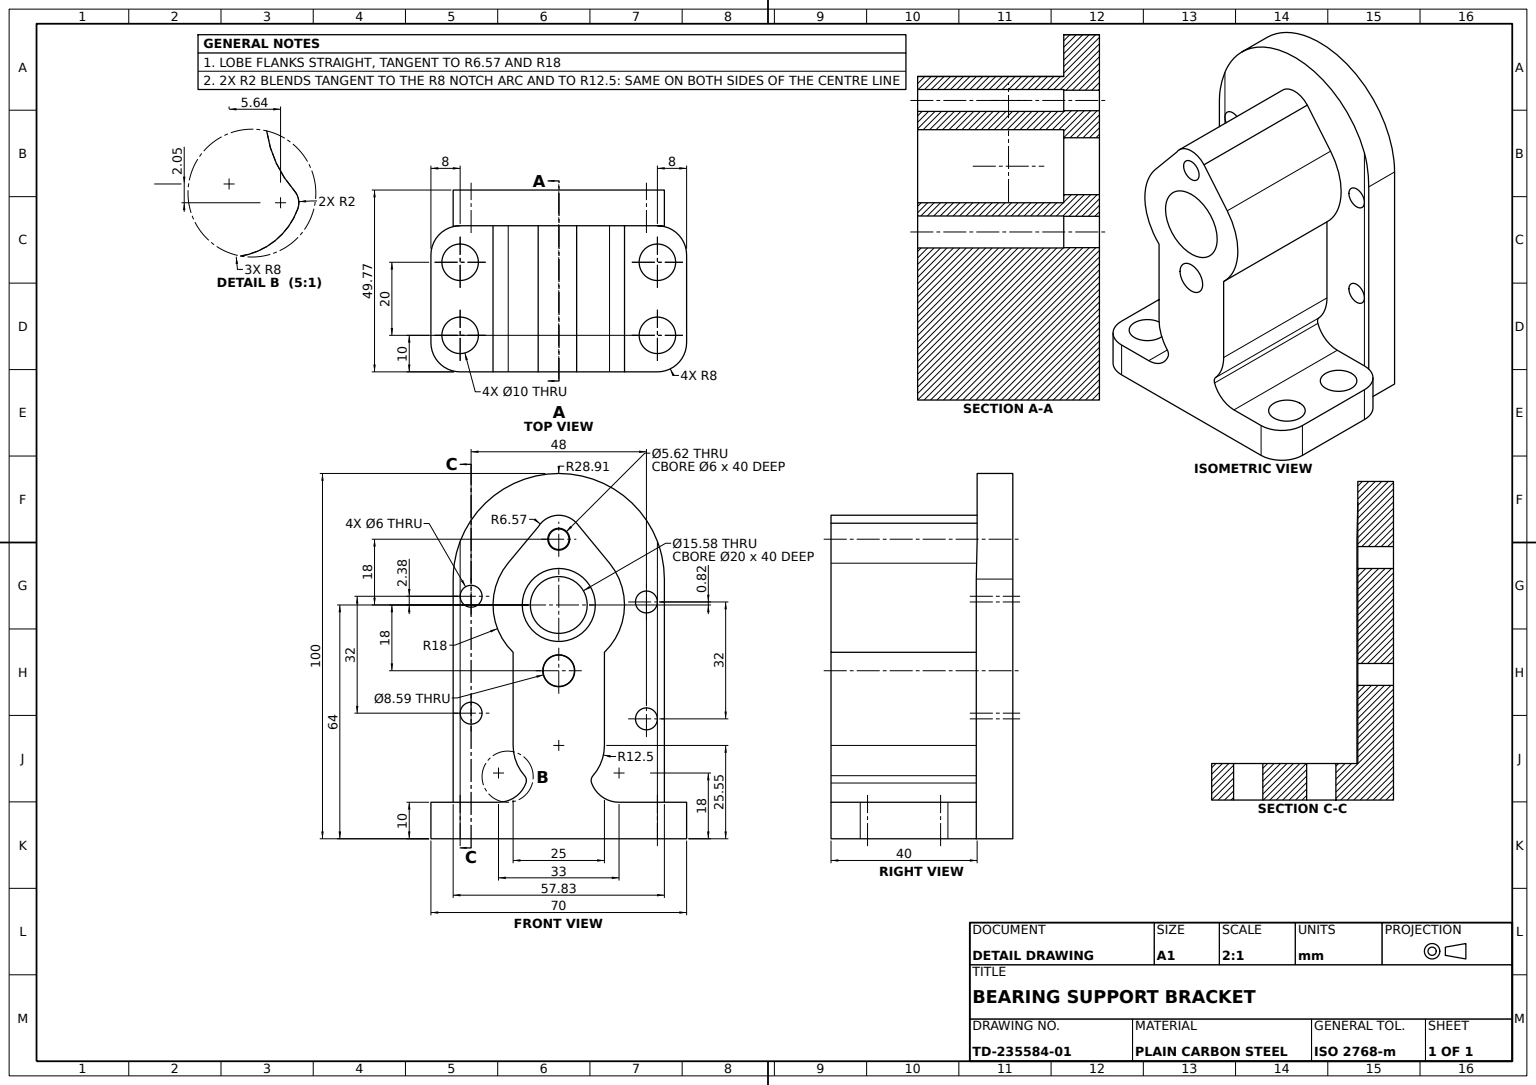
from build123d import *

# Parameters (mm, degrees)
BASE_PLATE_AND_COLUMN_SKETCH_R = 5
BASE_PLATE_AND_COLUMN_SKETCH_W = 18
BASE_PLATE_AND_COLUMN_SKETCH_H = 40
BASE_PLATE_DEPTH               = 10
FRONT_PROFILE_SKETCH_R         = 4.377272593
FRONT_PROFILE_BOSS_40MM_DEPTH  = 40
UPRIGHT_COLUMN_100MM_DEPTH     = 100
COLUMN_EDGE_FILLETS_RADIUS     = 28.912605022
COLUMN_EDGE_FILLETS_LENGTH     = 10
SKETCH2_6_R                    = 4.295746386
SKETCH2_6_R_2                  = 7.787765557
SKETCH2_6_R_3                  = 2.809047726
THROUGH_CUT_A_DEPTH            = 100
SKETCH2_7_R                    = 3
THROUGH_CUT_B_DEPTH            = 100


with BuildPart() as part:
    # Base Plate and Column Sketch → Base Plate (new body)
    # profile 1 of 4: a face of its own
    with BuildSketch(Plane(origin=(0, 0, 0), x_dir=(1, 0, 0), z_dir=(0, 1, 0))):
        with BuildLine():
            Line((53, 40), (53, 0))
            Line((53, 0), (62, 0))
            ThreePointArc((62, 0), (67.656854249, 2.343145751), (70, 8))
            Line((70, 8), (70, 32))
            ThreePointArc((70, 32), (68.296857954, 36.934529351), (63.912605022, 39.768007597))
            ThreePointArc((63.912605022, 39.768007597), (62.963311793, 39.941790125), (62, 40))
            Line((62, 40), (53, 40))
        make_face()
        with Locations(Location((62, 10, 0), (0, 0, 270))):
            Circle(BASE_PLATE_AND_COLUMN_SKETCH_R, mode=Mode.SUBTRACT)
        with Locations(Location((62, 30, 0), (0, 0, 270))):
            Circle(BASE_PLATE_AND_COLUMN_SKETCH_R, mode=Mode.SUBTRACT)
    # profile 2 of 4: a face of its own
    with BuildSketch(Plane(origin=(0, 0, 0), x_dir=(1, 0, 0), z_dir=(0, 1, 0))):
        with BuildLine():
            ThreePointArc((0, 8), (2.343145751, 2.343145751), (8, 0))
            Line((8, 0), (17, 0))
            Line((17, 0), (17, 40))
            Line((17, 40), (8, 40))
            ThreePointArc((8, 40), (7.036688207, 39.941790125), (6.087394978, 39.768007597))
            ThreePointArc((6.087394978, 39.768007597), (1.703142046, 36.934529351), (0, 32))
            Line((0, 32), (0, 8))
        make_face()
        with Locations(Location((8, 10, 0), (0, 0, 270))):
            Circle(BASE_PLATE_AND_COLUMN_SKETCH_R, mode=Mode.SUBTRACT)
        with Locations(Location((8, 30, 0), (0, 0, 270))):
            Circle(BASE_PLATE_AND_COLUMN_SKETCH_R, mode=Mode.SUBTRACT)
    # profile 3 of 4: a face of its own
    with BuildSketch(Plane(origin=(0, 0, 0), x_dir=(1, 0, 0), z_dir=(0, 1, 0))):
        with Locations((26, 20)):
            Rectangle(BASE_PLATE_AND_COLUMN_SKETCH_W, BASE_PLATE_AND_COLUMN_SKETCH_H)
    # profile 4 of 4: a face of its own
    with BuildSketch(Plane(origin=(0, 0, 0), x_dir=(1, 0, 0), z_dir=(0, 1, 0))):
        with Locations((44, 20)):
            Rectangle(BASE_PLATE_AND_COLUMN_SKETCH_W, BASE_PLATE_AND_COLUMN_SKETCH_H)
    extrude(amount=BASE_PLATE_DEPTH)

    # Front Profile Sketch → Front Profile Boss 40mm (add)
    with BuildSketch(Plane.XY):
        with BuildLine():
            ThreePointArc((26.016312226, 15.260465273), (23.087140841, 11.445754131), (18.5, 10))
            Line((18.5, 10), (51.5, 10))
            ThreePointArc((51.5, 10), (46.912859159, 11.445754131), (43.983687774, 15.260465273))
            ThreePointArc((43.983687774, 15.260465273), (43.897725001, 16.317658687), (44.364453302, 17.270135567))
            ThreePointArc((44.364453302, 17.270135567), (46.68986027, 21.123183149), (47.5, 25.550051892))
            Line((47.5, 25.550051892), (47.5, 51.048166153))
            ThreePointArc((47.5, 51.048166153), (52.970478526, 62.969513929), (48.898595899, 75.438051934))
            Line((48.898595899, 75.438051934), (39.895129219, 86.378336678))
            ThreePointArc((39.895129219, 86.378336678), (34.372816044, 88.537489), (29.361733435, 85.367799323))
            Line((29.361733435, 85.367799323), (21.162337749, 75.511694203))
            ThreePointArc((21.162337749, 75.511694203), (17.026848791, 63.017230636), (22.5, 51.048166153))
            Line((22.5, 51.048166153), (22.5, 25.550051892))
            ThreePointArc((22.5, 25.550051892), (23.31013973, 21.123183149), (25.635546698, 17.270135567))
            ThreePointArc((25.635546698, 17.270135567), (26.102274999, 16.317658687), (26.016312226, 15.260465273))
        make_face()
        with Locations((35, 46)):
            Circle(FRONT_PROFILE_SKETCH_R, mode=Mode.SUBTRACT)
        with BuildLine():
            Line((34.943116214, 73.99983821), (34.943118802, 74.000202219))
            ThreePointArc((34.943118802, 74.000202219), (34.971559221, 74.000050555), (35, 74))
            ThreePointArc((35, 74), (42.071067812, 71.071067812), (45, 64))
            ThreePointArc((45, 64), (27.949072326, 56.908849252), (34.943116214, 73.99983821))
        make_face(mode=Mode.SUBTRACT)
        with BuildLine():
            ThreePointArc((38, 82), (37.113765438, 79.871151562), (34.978669551, 79.000075832))
            ThreePointArc((34.978669551, 79.000075832), (32.000018958, 82.010665292), (35, 85))
            ThreePointArc((35, 85), (37.121320344, 84.121320344), (38, 82))
        make_face(mode=Mode.SUBTRACT)
    extrude(amount=-FRONT_PROFILE_BOSS_40MM_DEPTH)

    # Sketch1_3 → Upright Column 100mm (add)
    with BuildSketch(Plane(origin=(0, 0, 0), x_dir=(1, 0, 0), z_dir=(0, 1, 0))):
        with BuildLine():
            Line((8, 40), (17, 40))
            Line((17, 40), (53, 40))
            Line((53, 40), (62, 40))
            ThreePointArc((62, 40), (62.963311793, 39.941790125), (63.912605022, 39.768007597))
            Line((63.912605022, 39.768007597), (63.912605022, 49.768007597))
            Line((63.912605022, 49.768007597), (6.087394978, 49.768007597))
            Line((6.087394978, 49.768007597), (6.087394978, 39.768007597))
            ThreePointArc((6.087394978, 39.768007597), (7.036688207, 39.941790125), (8, 40))
        make_face()
    extrude(amount=UPRIGHT_COLUMN_100MM_DEPTH)

    # Column Edge Fillets: full round fillet: the end face becomes a half cylinder, R = half its width
    column_edge_fillets_face = Plane((35, 100, -44.768007597), x_dir=(0, 0, 1), z_dir=(0, 1, 0))  # on the end face: x along it, z out of the body
    column_edge_fillets_slab = column_edge_fillets_face.offset(-COLUMN_EDGE_FILLETS_RADIUS / 2) * Box(COLUMN_EDGE_FILLETS_LENGTH, 2 * COLUMN_EDGE_FILLETS_RADIUS, COLUMN_EDGE_FILLETS_RADIUS, mode=Mode.PRIVATE)  # the body's end, R deep
    column_edge_fillets_round = Plane((35, 71.087394978, -44.768007597), x_dir=(0, 1, 0), z_dir=(0, 0, 1)) * Cylinder(COLUMN_EDGE_FILLETS_RADIUS, COLUMN_EDGE_FILLETS_LENGTH, mode=Mode.PRIVATE)  # its axis R under the face
    add(column_edge_fillets_slab - column_edge_fillets_round, mode=Mode.SUBTRACT)

    # Sketch2_6 → Through Cut A (cut)
    with BuildSketch(Plane.XY):
        with Locations((35, 46)):
            Circle(SKETCH2_6_R)
        with Locations((35, 64)):
            Circle(SKETCH2_6_R_2)
        with Locations((35, 82)):
            Circle(SKETCH2_6_R_3)
    extrude(amount=-THROUGH_CUT_A_DEPTH, mode=Mode.SUBTRACT)

    # Sketch2_7 → Through Cut B (cut)
    with BuildSketch(Plane.XY):
        with Locations((59, 64.824567346)):
            Circle(SKETCH2_7_R)
        with Locations((59, 32.824567346)):
            Circle(SKETCH2_7_R)
        with Locations(Location((11, 34.383225645, 0), (0, 0, 180))):
            Circle(SKETCH2_7_R)
        with Locations(Location((11, 66.383225645, 0), (0, 0, 180))):
            Circle(SKETCH2_7_R)
    extrude(amount=-THROUGH_CUT_B_DEPTH, mode=Mode.SUBTRACT)


solid = part.part
